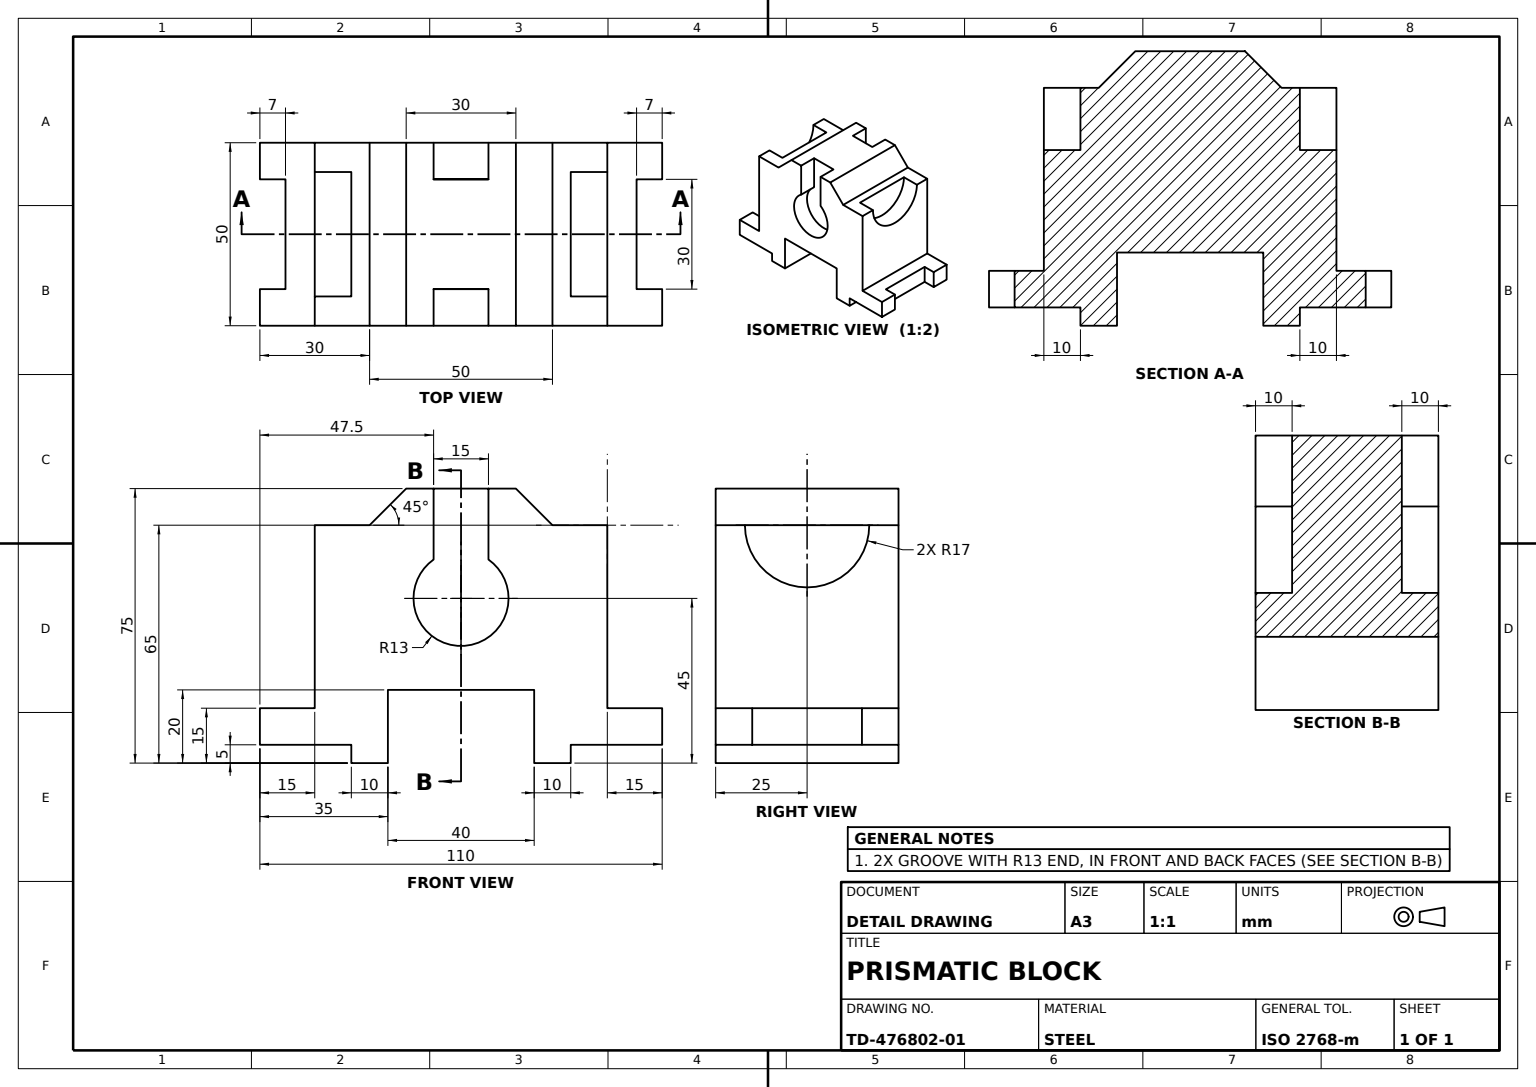
from build123d import *

# Parameters (mm, degrees)
MAIN_BODY_50MM_DEPTH     = 50
BEARING_SEAT_CUT_1_DEPTH = 10
BEARING_START            = -10
BEARING_SEAT_CUT_2_DEPTH = 10
TOP_GROOVE_CUT_1_DEPTH   = 10
TOP_START                = -10
TOP_GROOVE_CUT_2_DEPTH   = 10
BASE_NOTCH_1_SKETCH_W    = 7
BASE_NOTCH_1_SKETCH_H    = 30
BASE_NOTCH_CUT_1_DEPTH   = 10
BASE_NOTCH_2_SKETCH_W    = 7
BASE_NOTCH_2_SKETCH_H    = 30
BASE_NOTCH_CUT_2_DEPTH   = 10


with BuildPart() as part:
    # Body Profile Sketch → Main Body 50mm (new body)
    with BuildSketch(Plane.XY):
        Polygon((0, 0), (0, 5), (-25, 5), (-25, 15), (-10, 15), (-10, 65), (5, 65), (15, 75), (22.5, 75), (30, 75), (37.5, 75), (45, 75), (55, 65), (70, 65), (70, 15), (85, 15), (85, 5), (60, 5), (60, 0), (50, 0), (50, 20), (10, 20), (10, 0), align=None)
    extrude(amount=MAIN_BODY_50MM_DEPTH)

    # Bearing Seat 1 Sketch → Bearing Seat Cut 1 (cut)
    with BuildSketch(Plane.ZY.offset(10)):
        with BuildLine():
            Line((8, 65), (42, 65))
            ThreePointArc((42, 65), (25, 48), (8, 65))
        make_face()
    extrude(amount=-BEARING_SEAT_CUT_1_DEPTH, mode=Mode.SUBTRACT)

    # Bearing Seat 2 Sketch → Bearing Seat Cut 2 (cut)
    with BuildSketch(Plane(origin=(70, 0, 0), x_dir=(0, 0, -1), z_dir=(1, 0, 0)).offset(BEARING_START)):
        with BuildLine():
            Line((-42, 65), (-8, 65))
            ThreePointArc((-8, 65), (-25, 48), (-42, 65))
        make_face()
    extrude(amount=BEARING_SEAT_CUT_2_DEPTH, mode=Mode.SUBTRACT)

    # Top Groove 1 Sketch → Top Groove Cut 1 (cut)
    with BuildSketch(Plane(origin=(0, 0, 0), x_dir=(-1, 0, 0), z_dir=(0, 0, -1))):
        with BuildLine():
            Line((-30, 75), (-37.5, 75))
            Line((-37.5, 75), (-37.5, 55.618380291))
            ThreePointArc((-37.5, 55.618380291), (-30, 32), (-22.5, 55.618380291))
            Line((-22.5, 55.618380291), (-22.5, 75))
            Line((-22.5, 75), (-30, 75))
        make_face()
    extrude(amount=-TOP_GROOVE_CUT_1_DEPTH, mode=Mode.SUBTRACT)

    # Top Groove 2 Sketch → Top Groove Cut 2 (cut)
    with BuildSketch(Plane.XY.offset(50).offset(TOP_START)):
        with BuildLine():
            Line((30, 75), (22.5, 75))
            Line((22.5, 75), (22.5, 55.618380291))
            ThreePointArc((22.5, 55.618380291), (30, 32), (37.5, 55.618380291))
            Line((37.5, 55.618380291), (37.5, 75))
            Line((37.5, 75), (30, 75))
        make_face()
    extrude(amount=TOP_GROOVE_CUT_2_DEPTH, mode=Mode.SUBTRACT)

    # Base Notch 1 Sketch → Base Notch Cut 1 (cut)
    with BuildSketch(Plane(origin=(0, 15, 0), x_dir=(1, 0, 0), z_dir=(0, 1, 0))):
        with Locations((-21.5, -25)):
            Rectangle(BASE_NOTCH_1_SKETCH_W, BASE_NOTCH_1_SKETCH_H)
    extrude(amount=-BASE_NOTCH_CUT_1_DEPTH, mode=Mode.SUBTRACT)

    # Base Notch 2 Sketch → Base Notch Cut 2 (cut)
    with BuildSketch(Plane(origin=(0, 15, 0), x_dir=(1, 0, 0), z_dir=(0, 1, 0))):
        with Locations((81.5, -25)):
            Rectangle(BASE_NOTCH_2_SKETCH_W, BASE_NOTCH_2_SKETCH_H)
    extrude(amount=-BASE_NOTCH_CUT_2_DEPTH, mode=Mode.SUBTRACT)


solid = part.part
